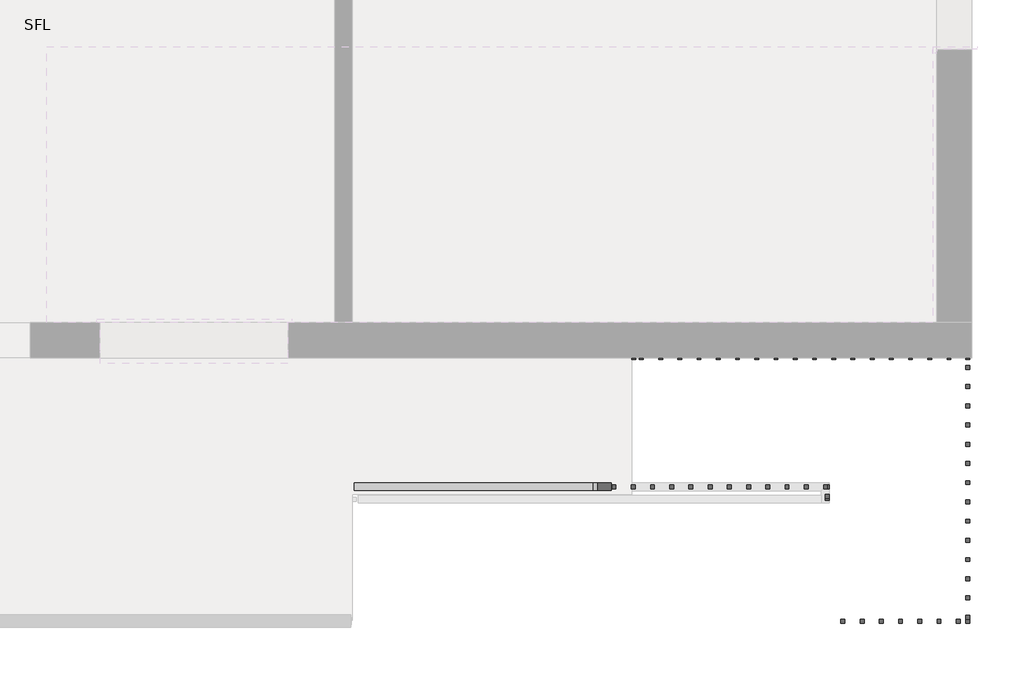
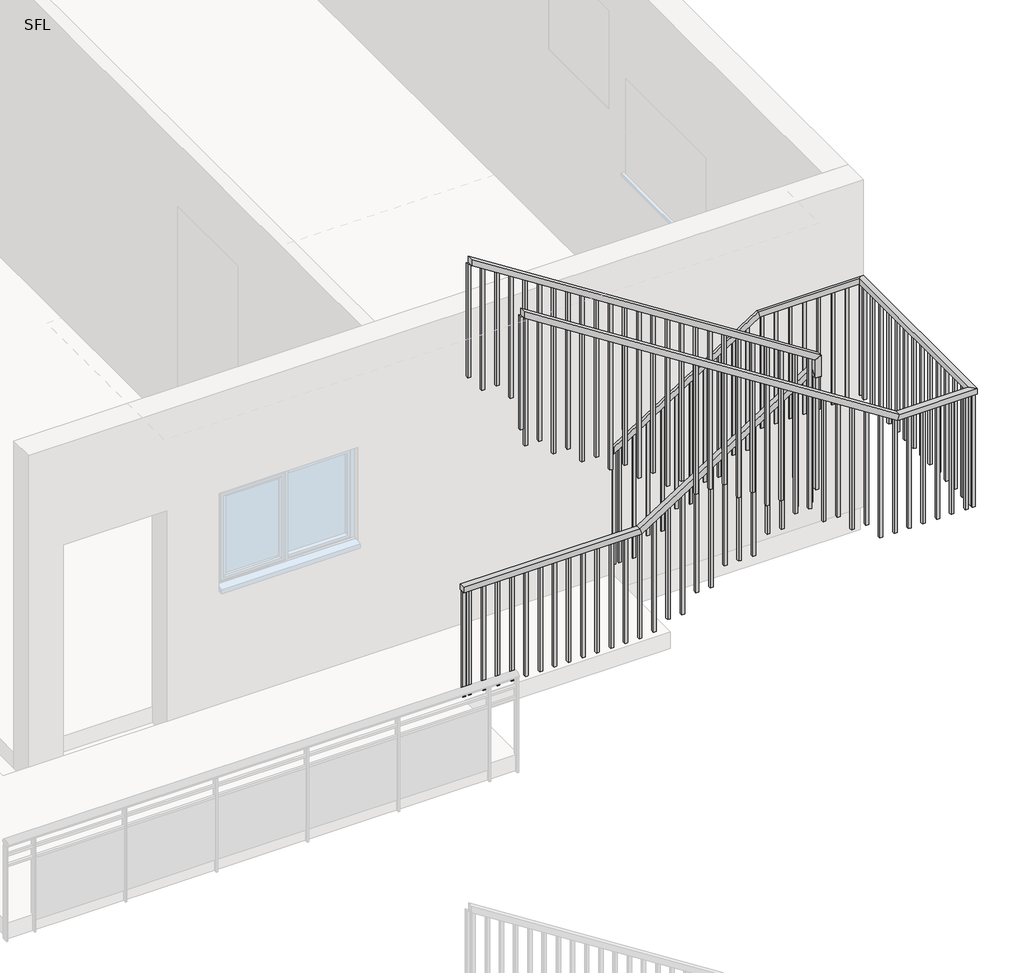
# One storey, part 3 of 4: 2 railings.
"""IFC4 building model written with IfcOpenShell, lengths in millimetres."""

from ifc_helpers import new_model, si_unit, frame, origin, place, context, project, spatial, polyline, outline, extrude, faceted_brep, element, save

model = new_model("IFC4")

# Units and contexts
model_context = context("Model", 3, world=origin())
ifc_project = project(units=[si_unit("LENGTHUNIT", "METRE", prefix="MILLI")], contexts=[model_context])

# Site, building, storey
site = spatial("IfcSite", under=ifc_project)
building = spatial("IfcBuilding", under=site)
storey = spatial("IfcBuildingStorey", under=building, Name="SFL", Elevation=6583.68)

# Railings
placement = place(None, origin())
element("IfcRailing", 1, ObjectType="1100mm", at=placement, inside=storey, context=model_context, shape_type="SolidModel", body=[
    faceted_brep([(-8680.149573, -10194.6521308, 7927.52), (-8680.149573, -10194.6521308, 7868.1623995), (-8680.149573, -10244.6521308, 7868.1623995), (-8680.149573, -10244.6521308, 7927.52), (-7409.7306254, -10194.6521308, 8740.32), (-7395.1045513, -10194.6521308, 8690.32), (-7395.1045513, -10244.6521308, 8690.32), (-7409.7306254, -10244.6521308, 8740.32), (-6470.4132565, -10194.6521308, 8740.32), (-6470.4132565, -10194.6521308, 8690.32), (-6520.4132565, -10244.6521308, 8690.32), (-6520.4132565, -10244.6521308, 8740.32), (-6470.4132565, -11959.0860066, 8740.32), (-6470.4132565, -11959.0860066, 8690.32), (-6520.4132565, -11909.0860066, 8690.32), (-6520.4132565, -11909.0860066, 8740.32), (-7155.718398, -11959.0860066, 8740.32), (-7170.3479429, -11959.0860066, 8690.32), (-7170.3479429, -11909.0860066, 8690.32), (-7155.718398, -11909.0860066, 8740.32), (-10457.8773536, -11959.0860066, 10853.6), (-10457.8773536, -11909.0860066, 10853.6), (-10457.8773536, -11909.0860066, 10794.237542), (-10457.8773536, -11959.0860066, 10794.237542)], [[[0, 1, 2, 3]], [[1, 0, 4, 5]], [[2, 1, 5, 6]], [[3, 2, 6, 7]], [[0, 3, 7, 4]], [[5, 4, 8, 9]], [[6, 5, 9, 10]], [[7, 6, 10, 11]], [[4, 7, 11, 8]], [[9, 8, 12, 13]], [[10, 9, 13, 14]], [[11, 10, 14, 15]], [[8, 11, 15, 12]], [[13, 12, 16, 17]], [[14, 13, 17, 18]], [[15, 14, 18, 19]], [[12, 15, 19, 16]], [[20, 21, 22, 23]], [[17, 16, 20, 23]], [[18, 17, 23, 22]], [[19, 18, 22, 21]], [[16, 19, 21, 20]]]),
    extrude(outline(polyline([(9591.04, -10420.4132565), (10770.2616741, -10420.4132565), (10786.2609039, -10445.4132565), (9591.04, -10445.4132565), (9591.04, -10420.4132565)])), frame((0.0, -11946.5860066, 0.0), z_axis=(0.0, 1.0, 0.0), x_axis=(0.0, 0.0, 1.0)), (0.0, 0.0, 1.0), 25.0),
    extrude(outline(polyline([(9591.04, -10295.4132565), (10690.265525, -10295.4132565), (10706.2647548, -10320.4132565), (9591.04, -10320.4132565), (9591.04, -10295.4132565)])), frame((0.0, -11946.5860066, 0.0), z_axis=(0.0, 1.0, 0.0), x_axis=(0.0, 0.0, 1.0)), (0.0, 0.0, 1.0), 25.0),
    extrude(outline(polyline([(9428.48, -10170.4132565), (10610.269376, -10170.4132565), (10626.2686058, -10195.4132565), (9428.48, -10195.4132565), (9428.48, -10170.4132565)])), frame((0.0, -11946.5860066, 0.0), z_axis=(0.0, 1.0, 0.0), x_axis=(0.0, 0.0, 1.0)), (0.0, 0.0, 1.0), 25.0),
    extrude(outline(polyline([(9428.48, -10045.4132565), (10530.2732269, -10045.4132565), (10546.2724567, -10070.4132565), (9428.48, -10070.4132565), (9428.48, -10045.4132565)])), frame((0.0, -11946.5860066, 0.0), z_axis=(0.0, 1.0, 0.0), x_axis=(0.0, 0.0, 1.0)), (0.0, 0.0, 1.0), 25.0),
    extrude(outline(polyline([(9265.92, -9920.4132565), (10450.2770779, -9920.4132565), (10466.2763077, -9945.4132565), (9265.92, -9945.4132565), (9265.92, -9920.4132565)])), frame((0.0, -11946.5860066, 0.0), z_axis=(0.0, 1.0, 0.0), x_axis=(0.0, 0.0, 1.0)), (0.0, 0.0, 1.0), 25.0),
    extrude(outline(polyline([(9265.92, -9795.4132565), (10370.2809288, -9795.4132565), (10386.2801586, -9820.4132565), (9265.92, -9820.4132565), (9265.92, -9795.4132565)])), frame((0.0, -11946.5860066, 0.0), z_axis=(0.0, 1.0, 0.0), x_axis=(0.0, 0.0, 1.0)), (0.0, 0.0, 1.0), 25.0),
    extrude(outline(polyline([(9103.36, -9670.4132565), (10290.2847798, -9670.4132565), (10306.2840096, -9695.4132565), (9103.36, -9695.4132565), (9103.36, -9670.4132565)])), frame((0.0, -11946.5860066, 0.0), z_axis=(0.0, 1.0, 0.0), x_axis=(0.0, 0.0, 1.0)), (0.0, 0.0, 1.0), 25.0),
    extrude(outline(polyline([(9103.36, -9545.4132565), (10210.2886307, -9545.4132565), (10226.2878605, -9570.4132565), (9103.36, -9570.4132565), (9103.36, -9545.4132565)])), frame((0.0, -11946.5860066, 0.0), z_axis=(0.0, 1.0, 0.0), x_axis=(0.0, 0.0, 1.0)), (0.0, 0.0, 1.0), 25.0),
    extrude(outline(polyline([(8940.8, -9420.4132565), (10130.2924817, -9420.4132565), (10146.2917115, -9445.4132565), (8940.8, -9445.4132565), (8940.8, -9420.4132565)])), frame((0.0, -11946.5860066, 0.0), z_axis=(0.0, 1.0, 0.0), x_axis=(0.0, 0.0, 1.0)), (0.0, 0.0, 1.0), 25.0),
    extrude(outline(polyline([(8940.8, -9295.4132565), (10050.2963326, -9295.4132565), (10066.2955624, -9320.4132565), (8940.8, -9320.4132565), (8940.8, -9295.4132565)])), frame((0.0, -11946.5860066, 0.0), z_axis=(0.0, 1.0, 0.0), x_axis=(0.0, 0.0, 1.0)), (0.0, 0.0, 1.0), 25.0),
    extrude(outline(polyline([(8778.24, -9170.4132565), (9970.3001836, -9170.4132565), (9986.2994134, -9195.4132565), (8778.24, -9195.4132565), (8778.24, -9170.4132565)])), frame((0.0, -11946.5860066, 0.0), z_axis=(0.0, 1.0, 0.0), x_axis=(0.0, 0.0, 1.0)), (0.0, 0.0, 1.0), 25.0),
    extrude(outline(polyline([(8778.24, -9045.4132565), (9890.3040345, -9045.4132565), (9906.3032643, -9070.4132565), (8778.24, -9070.4132565), (8778.24, -9045.4132565)])), frame((0.0, -11946.5860066, 0.0), z_axis=(0.0, 1.0, 0.0), x_axis=(0.0, 0.0, 1.0)), (0.0, 0.0, 1.0), 25.0),
    extrude(outline(polyline([(8615.68, -8920.4132565), (9810.3078855, -8920.4132565), (9826.3071153, -8945.4132565), (8615.68, -8945.4132565), (8615.68, -8920.4132565)])), frame((0.0, -11946.5860066, 0.0), z_axis=(0.0, 1.0, 0.0), x_axis=(0.0, 0.0, 1.0)), (0.0, 0.0, 1.0), 25.0),
    extrude(outline(polyline([(8615.68, -8795.4132565), (9730.3117364, -8795.4132565), (9746.3109662, -8820.4132565), (8615.68, -8820.4132565), (8615.68, -8795.4132565)])), frame((0.0, -11946.5860066, 0.0), z_axis=(0.0, 1.0, 0.0), x_axis=(0.0, 0.0, 1.0)), (0.0, 0.0, 1.0), 25.0),
    extrude(outline(polyline([(8615.68, -8670.4132565), (9650.3155874, -8670.4132565), (9666.3148172, -8695.4132565), (8615.68, -8695.4132565), (8615.68, -8670.4132565)])), frame((0.0, -11946.5860066, 0.0), z_axis=(0.0, 1.0, 0.0), x_axis=(0.0, 0.0, 1.0)), (0.0, 0.0, 1.0), 25.0),
    extrude(outline(polyline([(8453.12, -8545.4132565), (9570.3194383, -8545.4132565), (9586.3186681, -8570.4132565), (8453.12, -8570.4132565), (8453.12, -8545.4132565)])), frame((0.0, -11946.5860066, 0.0), z_axis=(0.0, 1.0, 0.0), x_axis=(0.0, 0.0, 1.0)), (0.0, 0.0, 1.0), 25.0),
    extrude(outline(polyline([(8453.12, -8420.4132565), (9490.3232893, -8420.4132565), (9506.3225191, -8445.4132565), (8453.12, -8445.4132565), (8453.12, -8420.4132565)])), frame((0.0, -11946.5860066, 0.0), z_axis=(0.0, 1.0, 0.0), x_axis=(0.0, 0.0, 1.0)), (0.0, 0.0, 1.0), 25.0),
    extrude(outline(polyline([(8290.56, -8295.4132565), (9410.3271402, -8295.4132565), (9426.32637, -8320.4132565), (8290.56, -8320.4132565), (8290.56, -8295.4132565)])), frame((0.0, -11946.5860066, 0.0), z_axis=(0.0, 1.0, 0.0), x_axis=(0.0, 0.0, 1.0)), (0.0, 0.0, 1.0), 25.0),
    extrude(outline(polyline([(8290.56, -8170.4132565), (9330.3309911, -8170.4132565), (9346.330221, -8195.4132565), (8290.56, -8195.4132565), (8290.56, -8170.4132565)])), frame((0.0, -11946.5860066, 0.0), z_axis=(0.0, 1.0, 0.0), x_axis=(0.0, 0.0, 1.0)), (0.0, 0.0, 1.0), 25.0),
    extrude(outline(polyline([(8128.0, -8045.4132565), (9250.3348421, -8045.4132565), (9266.3340719, -8070.4132565), (8128.0, -8070.4132565), (8128.0, -8045.4132565)])), frame((0.0, -11946.5860066, 0.0), z_axis=(0.0, 1.0, 0.0), x_axis=(0.0, 0.0, 1.0)), (0.0, 0.0, 1.0), 25.0),
    extrude(outline(polyline([(8128.0, -7920.4132565), (9170.338693, -7920.4132565), (9186.3379229, -7945.4132565), (8128.0, -7945.4132565), (8128.0, -7920.4132565)])), frame((0.0, -11946.5860066, 0.0), z_axis=(0.0, 1.0, 0.0), x_axis=(0.0, 0.0, 1.0)), (0.0, 0.0, 1.0), 25.0),
    extrude(outline(polyline([(7965.44, -7795.4132565), (9090.342544, -7795.4132565), (9106.3417738, -7820.4132565), (7965.44, -7820.4132565), (7965.44, -7795.4132565)])), frame((0.0, -11946.5860066, 0.0), z_axis=(0.0, 1.0, 0.0), x_axis=(0.0, 0.0, 1.0)), (0.0, 0.0, 1.0), 25.0),
    extrude(outline(polyline([(7965.44, -7670.4132565), (9010.3463949, -7670.4132565), (9026.3456247, -7695.4132565), (7965.44, -7695.4132565), (7965.44, -7670.4132565)])), frame((0.0, -11946.5860066, 0.0), z_axis=(0.0, 1.0, 0.0), x_axis=(0.0, 0.0, 1.0)), (0.0, 0.0, 1.0), 25.0),
    extrude(outline(polyline([(7802.88, -7545.4132565), (8930.3502459, -7545.4132565), (8946.3494757, -7570.4132565), (7802.88, -7570.4132565), (7802.88, -7545.4132565)])), frame((0.0, -11946.5860066, 0.0), z_axis=(0.0, 1.0, 0.0), x_axis=(0.0, 0.0, 1.0)), (0.0, 0.0, 1.0), 25.0),
    extrude(outline(polyline([(7802.88, -7420.4132565), (8850.3540968, -7420.4132565), (8866.3533266, -7445.4132565), (7802.88, -7445.4132565), (7802.88, -7420.4132565)])), frame((0.0, -11946.5860066, 0.0), z_axis=(0.0, 1.0, 0.0), x_axis=(0.0, 0.0, 1.0)), (0.0, 0.0, 1.0), 25.0),
    extrude(outline(polyline([(7640.32, -7295.4132565), (8770.3579478, -7295.4132565), (8786.3571776, -7320.4132565), (7640.32, -7320.4132565), (7640.32, -7295.4132565)])), frame((0.0, -11946.5860066, 0.0), z_axis=(0.0, 1.0, 0.0), x_axis=(0.0, 0.0, 1.0)), (0.0, 0.0, 1.0), 25.0),
    extrude(outline(polyline([(7640.32, -7170.4132565), (8690.3617987, -7170.4132565), (8706.3610285, -7195.4132565), (7640.32, -7195.4132565), (7640.32, -7170.4132565)])), frame((0.0, -11946.5860066, 0.0), z_axis=(0.0, 1.0, 0.0), x_axis=(0.0, 0.0, 1.0)), (0.0, 0.0, 1.0), 25.0),
    extrude(outline(polyline([(-7045.4132565, -11921.5860066), (-7045.4132565, -11946.5860066), (-7070.4132565, -11946.5860066), (-7070.4132565, -11921.5860066), (-7045.4132565, -11921.5860066)])), frame((0.0, 0.0, 7640.32), z_axis=(0.0, 0.0, 1.0), x_axis=(1.0, 0.0, 0.0)), (0.0, 0.0, 1.0), 1050.0),
    extrude(outline(polyline([(-6920.4132565, -11921.5860066), (-6920.4132565, -11946.5860066), (-6945.4132565, -11946.5860066), (-6945.4132565, -11921.5860066), (-6920.4132565, -11921.5860066)])), frame((0.0, 0.0, 7640.32), z_axis=(0.0, 0.0, 1.0), x_axis=(1.0, 0.0, 0.0)), (0.0, 0.0, 1.0), 1050.0),
    extrude(outline(polyline([(-6795.4132565, -11921.5860066), (-6795.4132565, -11946.5860066), (-6820.4132565, -11946.5860066), (-6820.4132565, -11921.5860066), (-6795.4132565, -11921.5860066)])), frame((0.0, 0.0, 7640.32), z_axis=(0.0, 0.0, 1.0), x_axis=(1.0, 0.0, 0.0)), (0.0, 0.0, 1.0), 1050.0),
    extrude(outline(polyline([(-6670.4132565, -11921.5860066), (-6670.4132565, -11946.5860066), (-6695.4132565, -11946.5860066), (-6695.4132565, -11921.5860066), (-6670.4132565, -11921.5860066)])), frame((0.0, 0.0, 7640.32), z_axis=(0.0, 0.0, 1.0), x_axis=(1.0, 0.0, 0.0)), (0.0, 0.0, 1.0), 1050.0),
    extrude(outline(polyline([(-6545.4132565, -11921.5860066), (-6545.4132565, -11946.5860066), (-6570.4132565, -11946.5860066), (-6570.4132565, -11921.5860066), (-6545.4132565, -11921.5860066)])), frame((0.0, 0.0, 7640.32), z_axis=(0.0, 0.0, 1.0), x_axis=(1.0, 0.0, 0.0)), (0.0, 0.0, 1.0), 1050.0),
    extrude(outline(polyline([(-6507.9132565, -11894.6521308), (-6482.9132565, -11894.6521308), (-6482.9132565, -11919.6521308), (-6507.9132565, -11919.6521308), (-6507.9132565, -11894.6521308)])), frame((0.0, 0.0, 7640.32), z_axis=(0.0, 0.0, 1.0), x_axis=(1.0, 0.0, 0.0)), (0.0, 0.0, 1.0), 1050.0),
    extrude(outline(polyline([(-6507.9132565, -11769.6521308), (-6482.9132565, -11769.6521308), (-6482.9132565, -11794.6521308), (-6507.9132565, -11794.6521308), (-6507.9132565, -11769.6521308)])), frame((0.0, 0.0, 7640.32), z_axis=(0.0, 0.0, 1.0), x_axis=(1.0, 0.0, 0.0)), (0.0, 0.0, 1.0), 1050.0),
    extrude(outline(polyline([(-6507.9132565, -11644.6521308), (-6482.9132565, -11644.6521308), (-6482.9132565, -11669.6521308), (-6507.9132565, -11669.6521308), (-6507.9132565, -11644.6521308)])), frame((0.0, 0.0, 7640.32), z_axis=(0.0, 0.0, 1.0), x_axis=(1.0, 0.0, 0.0)), (0.0, 0.0, 1.0), 1050.0),
    extrude(outline(polyline([(-6507.9132565, -11519.6521308), (-6482.9132565, -11519.6521308), (-6482.9132565, -11544.6521308), (-6507.9132565, -11544.6521308), (-6507.9132565, -11519.6521308)])), frame((0.0, 0.0, 7640.32), z_axis=(0.0, 0.0, 1.0), x_axis=(1.0, 0.0, 0.0)), (0.0, 0.0, 1.0), 1050.0),
    extrude(outline(polyline([(-6507.9132565, -11394.6521308), (-6482.9132565, -11394.6521308), (-6482.9132565, -11419.6521308), (-6507.9132565, -11419.6521308), (-6507.9132565, -11394.6521308)])), frame((0.0, 0.0, 7640.32), z_axis=(0.0, 0.0, 1.0), x_axis=(1.0, 0.0, 0.0)), (0.0, 0.0, 1.0), 1050.0),
    extrude(outline(polyline([(-6507.9132565, -11269.6521308), (-6482.9132565, -11269.6521308), (-6482.9132565, -11294.6521308), (-6507.9132565, -11294.6521308), (-6507.9132565, -11269.6521308)])), frame((0.0, 0.0, 7640.32), z_axis=(0.0, 0.0, 1.0), x_axis=(1.0, 0.0, 0.0)), (0.0, 0.0, 1.0), 1050.0),
    extrude(outline(polyline([(-6507.9132565, -11144.6521308), (-6482.9132565, -11144.6521308), (-6482.9132565, -11169.6521308), (-6507.9132565, -11169.6521308), (-6507.9132565, -11144.6521308)])), frame((0.0, 0.0, 7640.32), z_axis=(0.0, 0.0, 1.0), x_axis=(1.0, 0.0, 0.0)), (0.0, 0.0, 1.0), 1050.0),
    extrude(outline(polyline([(-6507.9132565, -11019.6521308), (-6482.9132565, -11019.6521308), (-6482.9132565, -11044.6521308), (-6507.9132565, -11044.6521308), (-6507.9132565, -11019.6521308)])), frame((0.0, 0.0, 7640.32), z_axis=(0.0, 0.0, 1.0), x_axis=(1.0, 0.0, 0.0)), (0.0, 0.0, 1.0), 1050.0),
    extrude(outline(polyline([(-6507.9132565, -10894.6521308), (-6482.9132565, -10894.6521308), (-6482.9132565, -10919.6521308), (-6507.9132565, -10919.6521308), (-6507.9132565, -10894.6521308)])), frame((0.0, 0.0, 7640.32), z_axis=(0.0, 0.0, 1.0), x_axis=(1.0, 0.0, 0.0)), (0.0, 0.0, 1.0), 1050.0),
    extrude(outline(polyline([(-6507.9132565, -10769.6521308), (-6482.9132565, -10769.6521308), (-6482.9132565, -10794.6521308), (-6507.9132565, -10794.6521308), (-6507.9132565, -10769.6521308)])), frame((0.0, 0.0, 7640.32), z_axis=(0.0, 0.0, 1.0), x_axis=(1.0, 0.0, 0.0)), (0.0, 0.0, 1.0), 1050.0),
    extrude(outline(polyline([(-6507.9132565, -10644.6521308), (-6482.9132565, -10644.6521308), (-6482.9132565, -10669.6521308), (-6507.9132565, -10669.6521308), (-6507.9132565, -10644.6521308)])), frame((0.0, 0.0, 7640.32), z_axis=(0.0, 0.0, 1.0), x_axis=(1.0, 0.0, 0.0)), (0.0, 0.0, 1.0), 1050.0),
    extrude(outline(polyline([(-6507.9132565, -10519.6521308), (-6482.9132565, -10519.6521308), (-6482.9132565, -10544.6521308), (-6507.9132565, -10544.6521308), (-6507.9132565, -10519.6521308)])), frame((0.0, 0.0, 7640.32), z_axis=(0.0, 0.0, 1.0), x_axis=(1.0, 0.0, 0.0)), (0.0, 0.0, 1.0), 1050.0),
    extrude(outline(polyline([(-6507.9132565, -10394.6521308), (-6482.9132565, -10394.6521308), (-6482.9132565, -10419.6521308), (-6507.9132565, -10419.6521308), (-6507.9132565, -10394.6521308)])), frame((0.0, 0.0, 7640.32), z_axis=(0.0, 0.0, 1.0), x_axis=(1.0, 0.0, 0.0)), (0.0, 0.0, 1.0), 1050.0),
    extrude(outline(polyline([(-6507.9132565, -10269.6521308), (-6482.9132565, -10269.6521308), (-6482.9132565, -10294.6521308), (-6507.9132565, -10294.6521308), (-6507.9132565, -10269.6521308)])), frame((0.0, 0.0, 7640.32), z_axis=(0.0, 0.0, 1.0), x_axis=(1.0, 0.0, 0.0)), (0.0, 0.0, 1.0), 1050.0),
    extrude(outline(polyline([(-6630.149573, -10232.1521308), (-6630.149573, -10207.1521308), (-6605.149573, -10207.1521308), (-6605.149573, -10232.1521308), (-6630.149573, -10232.1521308)])), frame((0.0, 0.0, 7640.32), z_axis=(0.0, 0.0, 1.0), x_axis=(1.0, 0.0, 0.0)), (0.0, 0.0, 1.0), 1050.0),
    extrude(outline(polyline([(-6755.149573, -10232.1521308), (-6755.149573, -10207.1521308), (-6730.149573, -10207.1521308), (-6730.149573, -10232.1521308), (-6755.149573, -10232.1521308)])), frame((0.0, 0.0, 7640.32), z_axis=(0.0, 0.0, 1.0), x_axis=(1.0, 0.0, 0.0)), (0.0, 0.0, 1.0), 1050.0),
    extrude(outline(polyline([(-6880.149573, -10232.1521308), (-6880.149573, -10207.1521308), (-6855.149573, -10207.1521308), (-6855.149573, -10232.1521308), (-6880.149573, -10232.1521308)])), frame((0.0, 0.0, 7640.32), z_axis=(0.0, 0.0, 1.0), x_axis=(1.0, 0.0, 0.0)), (0.0, 0.0, 1.0), 1050.0),
    extrude(outline(polyline([(-7005.149573, -10232.1521308), (-7005.149573, -10207.1521308), (-6980.149573, -10207.1521308), (-6980.149573, -10232.1521308), (-7005.149573, -10232.1521308)])), frame((0.0, 0.0, 7640.32), z_axis=(0.0, 0.0, 1.0), x_axis=(1.0, 0.0, 0.0)), (0.0, 0.0, 1.0), 1050.0),
    extrude(outline(polyline([(-7130.149573, -10232.1521308), (-7130.149573, -10207.1521308), (-7105.149573, -10207.1521308), (-7105.149573, -10232.1521308), (-7130.149573, -10232.1521308)])), frame((0.0, 0.0, 7640.32), z_axis=(0.0, 0.0, 1.0), x_axis=(1.0, 0.0, 0.0)), (0.0, 0.0, 1.0), 1050.0),
    extrude(outline(polyline([(-7255.149573, -10232.1521308), (-7255.149573, -10207.1521308), (-7230.149573, -10207.1521308), (-7230.149573, -10232.1521308), (-7255.149573, -10232.1521308)])), frame((0.0, 0.0, 7640.32), z_axis=(0.0, 0.0, 1.0), x_axis=(1.0, 0.0, 0.0)), (0.0, 0.0, 1.0), 1050.0),
    extrude(outline(polyline([(-7380.149573, -10232.1521308), (-7380.149573, -10207.1521308), (-7355.149573, -10207.1521308), (-7355.149573, -10232.1521308), (-7380.149573, -10232.1521308)])), frame((0.0, 0.0, 7640.32), z_axis=(0.0, 0.0, 1.0), x_axis=(1.0, 0.0, 0.0)), (0.0, 0.0, 1.0), 1050.0),
    extrude(outline(polyline([(8619.9144115, -7505.149573), (7477.76, -7505.149573), (7477.76, -7480.149573), (8635.9091352, -7480.149573), (8619.9144115, -7505.149573)])), frame((0.0, -10232.1521308, 0.0), z_axis=(0.0, 1.0, 0.0), x_axis=(0.0, 0.0, 1.0)), (0.0, 0.0, 1.0), 25.0),
    extrude(outline(polyline([(8539.9407932, -7630.149573), (7477.76, -7630.149573), (7477.76, -7605.149573), (8555.9355169, -7605.149573), (8539.9407932, -7630.149573)])), frame((0.0, -10232.1521308, 0.0), z_axis=(0.0, 1.0, 0.0), x_axis=(0.0, 0.0, 1.0)), (0.0, 0.0, 1.0), 25.0),
    extrude(outline(polyline([(8459.9671749, -7755.149573), (7315.2, -7755.149573), (7315.2, -7730.149573), (8475.9618986, -7730.149573), (8459.9671749, -7755.149573)])), frame((0.0, -10232.1521308, 0.0), z_axis=(0.0, 1.0, 0.0), x_axis=(0.0, 0.0, 1.0)), (0.0, 0.0, 1.0), 25.0),
    extrude(outline(polyline([(8379.9935566, -7880.149573), (7315.2, -7880.149573), (7315.2, -7855.149573), (8395.9882803, -7855.149573), (8379.9935566, -7880.149573)])), frame((0.0, -10232.1521308, 0.0), z_axis=(0.0, 1.0, 0.0), x_axis=(0.0, 0.0, 1.0)), (0.0, 0.0, 1.0), 25.0),
    extrude(outline(polyline([(8300.0199383, -8005.149573), (7152.64, -8005.149573), (7152.64, -7980.149573), (8316.014662, -7980.149573), (8300.0199383, -8005.149573)])), frame((0.0, -10232.1521308, 0.0), z_axis=(0.0, 1.0, 0.0), x_axis=(0.0, 0.0, 1.0)), (0.0, 0.0, 1.0), 25.0),
    extrude(outline(polyline([(8220.04632, -8130.149573), (7152.64, -8130.149573), (7152.64, -8105.149573), (8236.0410437, -8105.149573), (8220.04632, -8130.149573)])), frame((0.0, -10232.1521308, 0.0), z_axis=(0.0, 1.0, 0.0), x_axis=(0.0, 0.0, 1.0)), (0.0, 0.0, 1.0), 25.0),
    extrude(outline(polyline([(8140.0727017, -8255.149573), (6990.08, -8255.149573), (6990.08, -8230.149573), (8156.0674254, -8230.149573), (8140.0727017, -8255.149573)])), frame((0.0, -10232.1521308, 0.0), z_axis=(0.0, 1.0, 0.0), x_axis=(0.0, 0.0, 1.0)), (0.0, 0.0, 1.0), 25.0),
    extrude(outline(polyline([(8060.0990834, -8380.149573), (6990.08, -8380.149573), (6990.08, -8355.149573), (8076.0938071, -8355.149573), (8060.0990834, -8380.149573)])), frame((0.0, -10232.1521308, 0.0), z_axis=(0.0, 1.0, 0.0), x_axis=(0.0, 0.0, 1.0)), (0.0, 0.0, 1.0), 25.0),
    extrude(outline(polyline([(7980.1254651, -8505.149573), (6827.52, -8505.149573), (6827.52, -8480.149573), (7996.1201888, -8480.149573), (7980.1254651, -8505.149573)])), frame((0.0, -10232.1521308, 0.0), z_axis=(0.0, 1.0, 0.0), x_axis=(0.0, 0.0, 1.0)), (0.0, 0.0, 1.0), 25.0),
    extrude(outline(polyline([(7900.1518468, -8630.149573), (6827.52, -8630.149573), (6827.52, -8605.149573), (7916.1465705, -8605.149573), (7900.1518468, -8630.149573)])), frame((0.0, -10232.1521308, 0.0), z_axis=(0.0, 1.0, 0.0), x_axis=(0.0, 0.0, 1.0)), (0.0, 0.0, 1.0), 25.0),
    extrude(outline(polyline([(-6507.9132565, -11921.5860066), (-6482.9132565, -11921.5860066), (-6482.9132565, -11946.5860066), (-6507.9132565, -11946.5860066), (-6507.9132565, -11921.5860066)])), frame((0.0, 0.0, 7640.32), z_axis=(0.0, 0.0, 1.0), x_axis=(1.0, 0.0, 0.0)), (0.0, 0.0, 1.0), 1050.0),
    extrude(outline(polyline([(-6507.9132565, -10232.1521308), (-6507.9132565, -10207.1521308), (-6482.9132565, -10207.1521308), (-6482.9132565, -10232.1521308), (-6507.9132565, -10232.1521308)])), frame((0.0, 0.0, 7640.32), z_axis=(0.0, 0.0, 1.0), x_axis=(1.0, 0.0, 0.0)), (0.0, 0.0, 1.0), 1050.0),
    extrude(outline(polyline([(9753.6, -10458.2132565), (10794.4525096, -10458.2132565), (10810.4517394, -10483.2132565), (9753.6, -10483.2132565), (9753.6, -10458.2132565)])), frame((0.0, -11946.5860066, 0.0), z_axis=(0.0, 1.0, 0.0), x_axis=(0.0, 0.0, 1.0)), (0.0, 0.0, 1.0), 25.0),
    extrude(outline(polyline([(7868.1623995, -8680.149573), (6827.52, -8680.149573), (6827.52, -8655.149573), (7884.1571231, -8655.149573), (7868.1623995, -8680.149573)])), frame((0.0, -10232.1521308, 0.0), z_axis=(0.0, 1.0, 0.0), x_axis=(0.0, 0.0, 1.0)), (0.0, 0.0, 1.0), 25.0),
])
element("IfcRailing", 2, ObjectType="1100mm", at=placement, inside=storey, context=model_context, shape_type="SolidModel", body=[
    faceted_brep([(-10483.1306254, -11033.3255223, 7764.96), (-10483.1306254, -11033.3255223, 7714.96), (-10483.1306254, -11083.3255223, 7714.96), (-10483.1306254, -11083.3255223, 7764.96), (-8934.2333625, -11033.3255223, 7764.96), (-8919.6072884, -11033.3255223, 7714.96), (-8919.6072884, -11083.3255223, 7714.96), (-8934.2333625, -11083.3255223, 7764.96), (-7434.7306254, -11033.3255223, 8724.3252763), (-7434.7306254, -11083.3255223, 8724.3252763), (-7434.7306254, -11083.3255223, 8664.9676758), (-7434.7306254, -11033.3255223, 8664.9676758)], [[[0, 1, 2, 3]], [[1, 0, 4, 5]], [[2, 1, 5, 6]], [[3, 2, 6, 7]], [[0, 3, 7, 4]], [[8, 9, 10, 11]], [[5, 4, 8, 11]], [[6, 5, 11, 10]], [[7, 6, 10, 9]], [[4, 7, 9, 8]]]),
    faceted_brep([(-7384.7306254, -11033.3255223, 8740.32), (-7384.7306254, -11033.3255223, 8690.32), (-7434.7306254, -11033.3255223, 8690.32), (-7434.7306254, -11033.3255223, 8740.32), (-7384.7306254, -11109.5255223, 8740.32), (-7434.7306254, -11109.5255223, 8740.32), (-7434.7306254, -11159.5255223, 8690.32), (-7384.7306254, -11159.5255223, 8690.32)], [[[0, 1, 2, 3]], [[4, 5, 6, 7]], [[1, 0, 4, 7]], [[2, 1, 7, 6]], [[3, 2, 6, 5]], [[0, 3, 5, 4]]]),
    faceted_brep([(-7384.7306254, -11109.5255223, 8740.32), (-7384.7306254, -11159.5255223, 8690.32), (-7434.7306254, -11159.5255223, 8690.32), (-7434.7306254, -11109.5255223, 8740.32), (-7384.7306254, -11109.5255223, 8886.8807702), (-7434.7306254, -11109.5255223, 8859.5167718), (-7434.7306254, -11159.5255223, 8859.5167718), (-7384.7306254, -11159.5255223, 8886.8807702)], [[[0, 1, 2, 3]], [[4, 5, 6, 7]], [[1, 0, 4, 7]], [[2, 1, 7, 6]], [[3, 2, 6, 5]], [[0, 3, 5, 4]]]),
    faceted_brep([(-7384.7306254, -11159.5255223, 8886.8807702), (-7434.7306254, -11159.5255223, 8859.5167718), (-7434.7306254, -11109.5255223, 8859.5167718), (-7384.7306254, -11109.5255223, 8886.8807702), (-10457.8773536, -11159.5255223, 10853.6), (-10457.8773536, -11109.5255223, 10853.6), (-10457.8773536, -11109.5255223, 10794.237542), (-10457.8773536, -11159.5255223, 10794.237542)], [[[0, 1, 2, 3]], [[4, 5, 6, 7]], [[1, 0, 4, 7]], [[2, 1, 7, 6]], [[3, 2, 6, 5]], [[0, 3, 5, 4]]]),
    extrude(outline(polyline([(9753.6, -10459.7306254), (10795.4235789, -10459.7306254), (10811.4228087, -10484.7306254), (9753.6, -10484.7306254), (9753.6, -10459.7306254)])), frame((0.0, -11147.0255223, 0.0), z_axis=(0.0, 1.0, 0.0), x_axis=(0.0, 0.0, 1.0)), (0.0, 0.0, 1.0), 25.0),
    extrude(outline(polyline([(9591.04, -10334.7306254), (10715.4274298, -10334.7306254), (10731.4266596, -10359.7306254), (9591.04, -10359.7306254), (9591.04, -10334.7306254)])), frame((0.0, -11147.0255223, 0.0), z_axis=(0.0, 1.0, 0.0), x_axis=(0.0, 0.0, 1.0)), (0.0, 0.0, 1.0), 25.0),
    extrude(outline(polyline([(9591.04, -10209.7306254), (10635.4312808, -10209.7306254), (10651.4305106, -10234.7306254), (9591.04, -10234.7306254), (9591.04, -10209.7306254)])), frame((0.0, -11147.0255223, 0.0), z_axis=(0.0, 1.0, 0.0), x_axis=(0.0, 0.0, 1.0)), (0.0, 0.0, 1.0), 25.0),
    extrude(outline(polyline([(9428.48, -10084.7306254), (10555.4351317, -10084.7306254), (10571.4343615, -10109.7306254), (9428.48, -10109.7306254), (9428.48, -10084.7306254)])), frame((0.0, -11147.0255223, 0.0), z_axis=(0.0, 1.0, 0.0), x_axis=(0.0, 0.0, 1.0)), (0.0, 0.0, 1.0), 25.0),
    extrude(outline(polyline([(9428.48, -9959.7306254), (10475.4389827, -9959.7306254), (10491.4382125, -9984.7306254), (9428.48, -9984.7306254), (9428.48, -9959.7306254)])), frame((0.0, -11147.0255223, 0.0), z_axis=(0.0, 1.0, 0.0), x_axis=(0.0, 0.0, 1.0)), (0.0, 0.0, 1.0), 25.0),
    extrude(outline(polyline([(9265.92, -9834.7306254), (10395.4428336, -9834.7306254), (10411.4420634, -9859.7306254), (9265.92, -9859.7306254), (9265.92, -9834.7306254)])), frame((0.0, -11147.0255223, 0.0), z_axis=(0.0, 1.0, 0.0), x_axis=(0.0, 0.0, 1.0)), (0.0, 0.0, 1.0), 25.0),
    extrude(outline(polyline([(9265.92, -9709.7306254), (10315.4466846, -9709.7306254), (10331.4459144, -9734.7306254), (9265.92, -9734.7306254), (9265.92, -9709.7306254)])), frame((0.0, -11147.0255223, 0.0), z_axis=(0.0, 1.0, 0.0), x_axis=(0.0, 0.0, 1.0)), (0.0, 0.0, 1.0), 25.0),
    extrude(outline(polyline([(9103.36, -9584.7306254), (10235.4505355, -9584.7306254), (10251.4497653, -9609.7306254), (9103.36, -9609.7306254), (9103.36, -9584.7306254)])), frame((0.0, -11147.0255223, 0.0), z_axis=(0.0, 1.0, 0.0), x_axis=(0.0, 0.0, 1.0)), (0.0, 0.0, 1.0), 25.0),
    extrude(outline(polyline([(9103.36, -9459.7306254), (10155.4543865, -9459.7306254), (10171.4536163, -9484.7306254), (9103.36, -9484.7306254), (9103.36, -9459.7306254)])), frame((0.0, -11147.0255223, 0.0), z_axis=(0.0, 1.0, 0.0), x_axis=(0.0, 0.0, 1.0)), (0.0, 0.0, 1.0), 25.0),
    extrude(outline(polyline([(8940.8, -9334.7306254), (10075.4582374, -9334.7306254), (10091.4574672, -9359.7306254), (8940.8, -9359.7306254), (8940.8, -9334.7306254)])), frame((0.0, -11147.0255223, 0.0), z_axis=(0.0, 1.0, 0.0), x_axis=(0.0, 0.0, 1.0)), (0.0, 0.0, 1.0), 25.0),
    extrude(outline(polyline([(8940.8, -9209.7306254), (9995.4620884, -9209.7306254), (10011.4613182, -9234.7306254), (8940.8, -9234.7306254), (8940.8, -9209.7306254)])), frame((0.0, -11147.0255223, 0.0), z_axis=(0.0, 1.0, 0.0), x_axis=(0.0, 0.0, 1.0)), (0.0, 0.0, 1.0), 25.0),
    extrude(outline(polyline([(8778.24, -9084.7306254), (9915.4659393, -9084.7306254), (9931.4651691, -9109.7306254), (8778.24, -9109.7306254), (8778.24, -9084.7306254)])), frame((0.0, -11147.0255223, 0.0), z_axis=(0.0, 1.0, 0.0), x_axis=(0.0, 0.0, 1.0)), (0.0, 0.0, 1.0), 25.0),
    extrude(outline(polyline([(8778.24, -8959.7306254), (9835.4697903, -8959.7306254), (9851.4690201, -8984.7306254), (8778.24, -8984.7306254), (8778.24, -8959.7306254)])), frame((0.0, -11147.0255223, 0.0), z_axis=(0.0, 1.0, 0.0), x_axis=(0.0, 0.0, 1.0)), (0.0, 0.0, 1.0), 25.0),
    extrude(outline(polyline([(8615.68, -8834.7306254), (9755.4736412, -8834.7306254), (9771.472871, -8859.7306254), (8615.68, -8859.7306254), (8615.68, -8834.7306254)])), frame((0.0, -11147.0255223, 0.0), z_axis=(0.0, 1.0, 0.0), x_axis=(0.0, 0.0, 1.0)), (0.0, 0.0, 1.0), 25.0),
    extrude(outline(polyline([(8615.68, -8709.7306254), (9675.4774922, -8709.7306254), (9691.476722, -8734.7306254), (8615.68, -8734.7306254), (8615.68, -8709.7306254)])), frame((0.0, -11147.0255223, 0.0), z_axis=(0.0, 1.0, 0.0), x_axis=(0.0, 0.0, 1.0)), (0.0, 0.0, 1.0), 25.0),
    extrude(outline(polyline([(8453.12, -8584.7306254), (9595.4813431, -8584.7306254), (9611.4805729, -8609.7306254), (8453.12, -8609.7306254), (8453.12, -8584.7306254)])), frame((0.0, -11147.0255223, 0.0), z_axis=(0.0, 1.0, 0.0), x_axis=(0.0, 0.0, 1.0)), (0.0, 0.0, 1.0), 25.0),
    extrude(outline(polyline([(8453.12, -8459.7306254), (9515.4851941, -8459.7306254), (9531.4844239, -8484.7306254), (8453.12, -8484.7306254), (8453.12, -8459.7306254)])), frame((0.0, -11147.0255223, 0.0), z_axis=(0.0, 1.0, 0.0), x_axis=(0.0, 0.0, 1.0)), (0.0, 0.0, 1.0), 25.0),
    extrude(outline(polyline([(8290.56, -8334.7306254), (9435.489045, -8334.7306254), (9451.4882748, -8359.7306254), (8290.56, -8359.7306254), (8290.56, -8334.7306254)])), frame((0.0, -11147.0255223, 0.0), z_axis=(0.0, 1.0, 0.0), x_axis=(0.0, 0.0, 1.0)), (0.0, 0.0, 1.0), 25.0),
    extrude(outline(polyline([(8290.56, -8209.7306254), (9355.3535566, -8209.7306254), (9371.3482803, -8234.7306254), (8290.56, -8234.7306254), (8290.56, -8209.7306254)])), frame((0.0, -11147.0255223, 0.0), z_axis=(0.0, 1.0, 0.0), x_axis=(0.0, 0.0, 1.0)), (0.0, 0.0, 1.0), 25.0),
    extrude(outline(polyline([(8128.0, -8084.7306254), (9275.3799383, -8084.7306254), (9291.374662, -8109.7306254), (8128.0, -8109.7306254), (8128.0, -8084.7306254)])), frame((0.0, -11147.0255223, 0.0), z_axis=(0.0, 1.0, 0.0), x_axis=(0.0, 0.0, 1.0)), (0.0, 0.0, 1.0), 25.0),
    extrude(outline(polyline([(8128.0, -7959.7306254), (9195.40632, -7959.7306254), (9211.4010437, -7984.7306254), (8128.0, -7984.7306254), (8128.0, -7959.7306254)])), frame((0.0, -11147.0255223, 0.0), z_axis=(0.0, 1.0, 0.0), x_axis=(0.0, 0.0, 1.0)), (0.0, 0.0, 1.0), 25.0),
    extrude(outline(polyline([(7965.44, -7834.7306254), (9115.4327017, -7834.7306254), (9131.4274254, -7859.7306254), (7965.44, -7859.7306254), (7965.44, -7834.7306254)])), frame((0.0, -11147.0255223, 0.0), z_axis=(0.0, 1.0, 0.0), x_axis=(0.0, 0.0, 1.0)), (0.0, 0.0, 1.0), 25.0),
    extrude(outline(polyline([(7965.44, -7709.7306254), (9035.4590834, -7709.7306254), (9051.4538071, -7734.7306254), (7965.44, -7734.7306254), (7965.44, -7709.7306254)])), frame((0.0, -11147.0255223, 0.0), z_axis=(0.0, 1.0, 0.0), x_axis=(0.0, 0.0, 1.0)), (0.0, 0.0, 1.0), 25.0),
    extrude(outline(polyline([(7802.88, -7584.7306254), (8955.4854651, -7584.7306254), (8971.4801888, -7609.7306254), (7802.88, -7609.7306254), (7802.88, -7584.7306254)])), frame((0.0, -11147.0255223, 0.0), z_axis=(0.0, 1.0, 0.0), x_axis=(0.0, 0.0, 1.0)), (0.0, 0.0, 1.0), 25.0),
    extrude(outline(polyline([(7802.88, -7459.7306254), (8875.5118468, -7459.7306254), (8891.5065705, -7484.7306254), (7802.88, -7484.7306254), (7802.88, -7459.7306254)])), frame((0.0, -11147.0255223, 0.0), z_axis=(0.0, 1.0, 0.0), x_axis=(0.0, 0.0, 1.0)), (0.0, 0.0, 1.0), 25.0),
    extrude(outline(polyline([(-7422.2306254, -11108.3255223), (-7397.2306254, -11108.3255223), (-7397.2306254, -11133.3255223), (-7422.2306254, -11133.3255223), (-7422.2306254, -11108.3255223)])), frame((0.0, 0.0, 7640.32), z_axis=(0.0, 0.0, 1.0), x_axis=(1.0, 0.0, 0.0)), (0.0, 0.0, 1.0), 1050.0),
    extrude(outline(polyline([(8665.9913381, -7433.1306254), (7477.76, -7433.1306254), (7477.76, -7408.1306254), (8681.9860618, -7408.1306254), (8665.9913381, -7433.1306254)])), frame((0.0, -11070.8255223, 0.0), z_axis=(0.0, 1.0, 0.0), x_axis=(0.0, 0.0, 1.0)), (0.0, 0.0, 1.0), 25.0),
    extrude(outline(polyline([(8586.0177198, -7558.1306254), (7477.76, -7558.1306254), (7477.76, -7533.1306254), (8602.0124435, -7533.1306254), (8586.0177198, -7558.1306254)])), frame((0.0, -11070.8255223, 0.0), z_axis=(0.0, 1.0, 0.0), x_axis=(0.0, 0.0, 1.0)), (0.0, 0.0, 1.0), 25.0),
    extrude(outline(polyline([(8506.0441015, -7683.1306254), (7315.2, -7683.1306254), (7315.2, -7658.1306254), (8522.0388252, -7658.1306254), (8506.0441015, -7683.1306254)])), frame((0.0, -11070.8255223, 0.0), z_axis=(0.0, 1.0, 0.0), x_axis=(0.0, 0.0, 1.0)), (0.0, 0.0, 1.0), 25.0),
    extrude(outline(polyline([(8426.0704832, -7808.1306254), (7315.2, -7808.1306254), (7315.2, -7783.1306254), (8442.0652069, -7783.1306254), (8426.0704832, -7808.1306254)])), frame((0.0, -11070.8255223, 0.0), z_axis=(0.0, 1.0, 0.0), x_axis=(0.0, 0.0, 1.0)), (0.0, 0.0, 1.0), 25.0),
    extrude(outline(polyline([(8346.0968649, -7933.1306254), (7152.64, -7933.1306254), (7152.64, -7908.1306254), (8362.0915886, -7908.1306254), (8346.0968649, -7933.1306254)])), frame((0.0, -11070.8255223, 0.0), z_axis=(0.0, 1.0, 0.0), x_axis=(0.0, 0.0, 1.0)), (0.0, 0.0, 1.0), 25.0),
    extrude(outline(polyline([(8266.1232466, -8058.1306254), (7152.64, -8058.1306254), (7152.64, -8033.1306254), (8282.1179703, -8033.1306254), (8266.1232466, -8058.1306254)])), frame((0.0, -11070.8255223, 0.0), z_axis=(0.0, 1.0, 0.0), x_axis=(0.0, 0.0, 1.0)), (0.0, 0.0, 1.0), 25.0),
    extrude(outline(polyline([(8186.1496283, -8183.1306254), (7152.64, -8183.1306254), (7152.64, -8158.1306254), (8202.144352, -8158.1306254), (8186.1496283, -8183.1306254)])), frame((0.0, -11070.8255223, 0.0), z_axis=(0.0, 1.0, 0.0), x_axis=(0.0, 0.0, 1.0)), (0.0, 0.0, 1.0), 25.0),
    extrude(outline(polyline([(8106.17601, -8308.1306254), (6990.08, -8308.1306254), (6990.08, -8283.1306254), (8122.1707337, -8283.1306254), (8106.17601, -8308.1306254)])), frame((0.0, -11070.8255223, 0.0), z_axis=(0.0, 1.0, 0.0), x_axis=(0.0, 0.0, 1.0)), (0.0, 0.0, 1.0), 25.0),
    extrude(outline(polyline([(8026.2023917, -8433.1306254), (6990.08, -8433.1306254), (6990.08, -8408.1306254), (8042.1971154, -8408.1306254), (8026.2023917, -8433.1306254)])), frame((0.0, -11070.8255223, 0.0), z_axis=(0.0, 1.0, 0.0), x_axis=(0.0, 0.0, 1.0)), (0.0, 0.0, 1.0), 25.0),
    extrude(outline(polyline([(7946.2287734, -8558.1306254), (6827.52, -8558.1306254), (6827.52, -8533.1306254), (7962.2234971, -8533.1306254), (7946.2287734, -8558.1306254)])), frame((0.0, -11070.8255223, 0.0), z_axis=(0.0, 1.0, 0.0), x_axis=(0.0, 0.0, 1.0)), (0.0, 0.0, 1.0), 25.0),
    extrude(outline(polyline([(7866.2551551, -8683.1306254), (6827.52, -8683.1306254), (6827.52, -8658.1306254), (7882.2498787, -8658.1306254), (7866.2551551, -8683.1306254)])), frame((0.0, -11070.8255223, 0.0), z_axis=(0.0, 1.0, 0.0), x_axis=(0.0, 0.0, 1.0)), (0.0, 0.0, 1.0), 25.0),
    extrude(outline(polyline([(7786.2815368, -8808.1306254), (6753.6364991, -8808.1306254), (6753.6364991, -8783.1306254), (7802.2762604, -8783.1306254), (7786.2815368, -8808.1306254)])), frame((0.0, -11070.8255223, 0.0), z_axis=(0.0, 1.0, 0.0), x_axis=(0.0, 0.0, 1.0)), (0.0, 0.0, 1.0), 25.0),
    extrude(outline(polyline([(7706.3079185, -8933.1306254), (6673.6628808, -8933.1306254), (6673.6628808, -8908.1306254), (7722.3026421, -8908.1306254), (7706.3079185, -8933.1306254)])), frame((0.0, -11070.8255223, 0.0), z_axis=(0.0, 1.0, 0.0), x_axis=(0.0, 0.0, 1.0)), (0.0, 0.0, 1.0), 25.0),
    extrude(outline(polyline([(-9058.1306254, -11070.8255223), (-9058.1306254, -11045.8255223), (-9033.1306254, -11045.8255223), (-9033.1306254, -11070.8255223), (-9058.1306254, -11070.8255223)])), frame((0.0, 0.0, 6664.96), z_axis=(0.0, 0.0, 1.0), x_axis=(1.0, 0.0, 0.0)), (0.0, 0.0, 1.0), 1050.0),
    extrude(outline(polyline([(-9183.1306254, -11070.8255223), (-9183.1306254, -11045.8255223), (-9158.1306254, -11045.8255223), (-9158.1306254, -11070.8255223), (-9183.1306254, -11070.8255223)])), frame((0.0, 0.0, 6664.96), z_axis=(0.0, 0.0, 1.0), x_axis=(1.0, 0.0, 0.0)), (0.0, 0.0, 1.0), 1050.0),
    extrude(outline(polyline([(-9308.1306254, -11070.8255223), (-9308.1306254, -11045.8255223), (-9283.1306254, -11045.8255223), (-9283.1306254, -11070.8255223), (-9308.1306254, -11070.8255223)])), frame((0.0, 0.0, 6664.96), z_axis=(0.0, 0.0, 1.0), x_axis=(1.0, 0.0, 0.0)), (0.0, 0.0, 1.0), 1050.0),
    extrude(outline(polyline([(-9433.1306254, -11070.8255223), (-9433.1306254, -11045.8255223), (-9408.1306254, -11045.8255223), (-9408.1306254, -11070.8255223), (-9433.1306254, -11070.8255223)])), frame((0.0, 0.0, 6664.96), z_axis=(0.0, 0.0, 1.0), x_axis=(1.0, 0.0, 0.0)), (0.0, 0.0, 1.0), 1050.0),
    extrude(outline(polyline([(-9558.1306254, -11070.8255223), (-9558.1306254, -11045.8255223), (-9533.1306254, -11045.8255223), (-9533.1306254, -11070.8255223), (-9558.1306254, -11070.8255223)])), frame((0.0, 0.0, 6664.96), z_axis=(0.0, 0.0, 1.0), x_axis=(1.0, 0.0, 0.0)), (0.0, 0.0, 1.0), 1050.0),
    extrude(outline(polyline([(-9683.1306254, -11070.8255223), (-9683.1306254, -11045.8255223), (-9658.1306254, -11045.8255223), (-9658.1306254, -11070.8255223), (-9683.1306254, -11070.8255223)])), frame((0.0, 0.0, 6664.96), z_axis=(0.0, 0.0, 1.0), x_axis=(1.0, 0.0, 0.0)), (0.0, 0.0, 1.0), 1050.0),
    extrude(outline(polyline([(-9808.1306254, -11070.8255223), (-9808.1306254, -11045.8255223), (-9783.1306254, -11045.8255223), (-9783.1306254, -11070.8255223), (-9808.1306254, -11070.8255223)])), frame((0.0, 0.0, 6664.96), z_axis=(0.0, 0.0, 1.0), x_axis=(1.0, 0.0, 0.0)), (0.0, 0.0, 1.0), 1050.0),
    extrude(outline(polyline([(-9933.1306254, -11070.8255223), (-9933.1306254, -11045.8255223), (-9908.1306254, -11045.8255223), (-9908.1306254, -11070.8255223), (-9933.1306254, -11070.8255223)])), frame((0.0, 0.0, 6664.96), z_axis=(0.0, 0.0, 1.0), x_axis=(1.0, 0.0, 0.0)), (0.0, 0.0, 1.0), 1050.0),
    extrude(outline(polyline([(-10058.1306254, -11070.8255223), (-10058.1306254, -11045.8255223), (-10033.1306254, -11045.8255223), (-10033.1306254, -11070.8255223), (-10058.1306254, -11070.8255223)])), frame((0.0, 0.0, 6664.96), z_axis=(0.0, 0.0, 1.0), x_axis=(1.0, 0.0, 0.0)), (0.0, 0.0, 1.0), 1050.0),
    extrude(outline(polyline([(-10183.1306254, -11070.8255223), (-10183.1306254, -11045.8255223), (-10158.1306254, -11045.8255223), (-10158.1306254, -11070.8255223), (-10183.1306254, -11070.8255223)])), frame((0.0, 0.0, 6664.96), z_axis=(0.0, 0.0, 1.0), x_axis=(1.0, 0.0, 0.0)), (0.0, 0.0, 1.0), 1050.0),
    extrude(outline(polyline([(-10308.1306254, -11070.8255223), (-10308.1306254, -11045.8255223), (-10283.1306254, -11045.8255223), (-10283.1306254, -11070.8255223), (-10308.1306254, -11070.8255223)])), frame((0.0, 0.0, 6664.96), z_axis=(0.0, 0.0, 1.0), x_axis=(1.0, 0.0, 0.0)), (0.0, 0.0, 1.0), 1050.0),
    extrude(outline(polyline([(-10433.1306254, -11070.8255223), (-10433.1306254, -11045.8255223), (-10408.1306254, -11045.8255223), (-10408.1306254, -11070.8255223), (-10433.1306254, -11070.8255223)])), frame((0.0, 0.0, 6664.96), z_axis=(0.0, 0.0, 1.0), x_axis=(1.0, 0.0, 0.0)), (0.0, 0.0, 1.0), 1050.0),
    extrude(outline(polyline([(-7422.2306254, -11122.0255223), (-7397.2306254, -11122.0255223), (-7397.2306254, -11147.0255223), (-7422.2306254, -11147.0255223), (-7422.2306254, -11122.0255223)])), frame((0.0, 0.0, 7640.32), z_axis=(0.0, 0.0, 1.0), x_axis=(1.0, 0.0, 0.0)), (0.0, 0.0, 1.0), 1050.0),
    extrude(outline(polyline([(8672.9650376, -7422.2306254), (7640.32, -7422.2306254), (7640.32, -7397.2306254), (8688.9597613, -7397.2306254), (8672.9650376, -7422.2306254)])), frame((0.0, -11070.8255223, 0.0), z_axis=(0.0, 1.0, 0.0), x_axis=(0.0, 0.0, 1.0)), (0.0, 0.0, 1.0), 25.0),
    extrude(outline(polyline([(9753.6, -10458.1306254), (10794.3996282, -10458.1306254), (10810.398858, -10483.1306254), (9753.6, -10483.1306254), (9753.6, -10458.1306254)])), frame((0.0, -11147.0255223, 0.0), z_axis=(0.0, 1.0, 0.0), x_axis=(0.0, 0.0, 1.0)), (0.0, 0.0, 1.0), 25.0),
    extrude(outline(polyline([(-10483.1306254, -11070.8255223), (-10483.1306254, -11045.8255223), (-10458.1306254, -11045.8255223), (-10458.1306254, -11070.8255223), (-10483.1306254, -11070.8255223)])), frame((0.0, 0.0, 6664.96), z_axis=(0.0, 0.0, 1.0), x_axis=(1.0, 0.0, 0.0)), (0.0, 0.0, 1.0), 1050.0),
])

save(model, "model.ifc")

# Revit data of these elements
# Type "1100mm"
#   built-in parameter 1008612 = 0.019685 (stored number, unit not read)
#   built-in parameter 1008611 = 0.019685 (stored number, unit not read)
#   built-in parameter 1008609 = 0.902231 (stored number, unit not read)
#   built-in parameter 1008604 = 0.19685 (stored number, unit not read)
#   built-in parameter 1008603 = 0.164042 (stored number, unit not read)
#   Railing Height = 3.608924 ft
#   built-in parameter 1008630 = 2
#   built-in parameter 1008610 = 2
#   built-in parameter 1008608 = 1
#   built-in parameter 1008618 = Baluster_Square : 25mm
# Elements 1, 2 (IfcRailing, "1100mm")
#   Phase Created = New Construction
